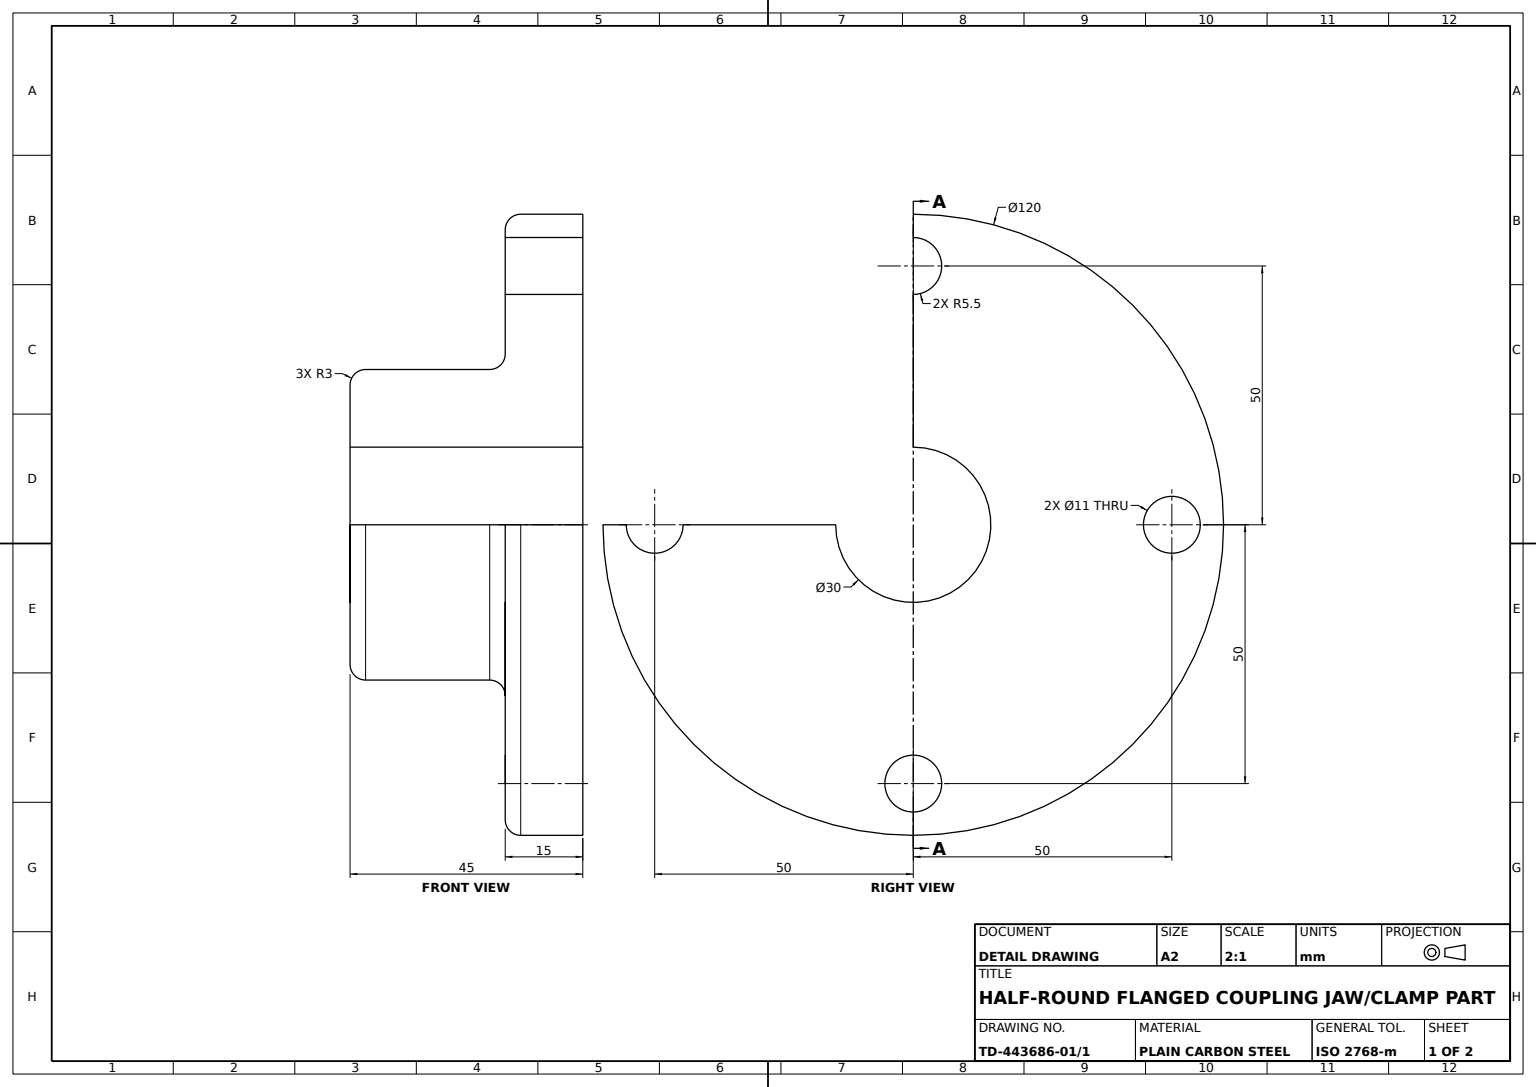
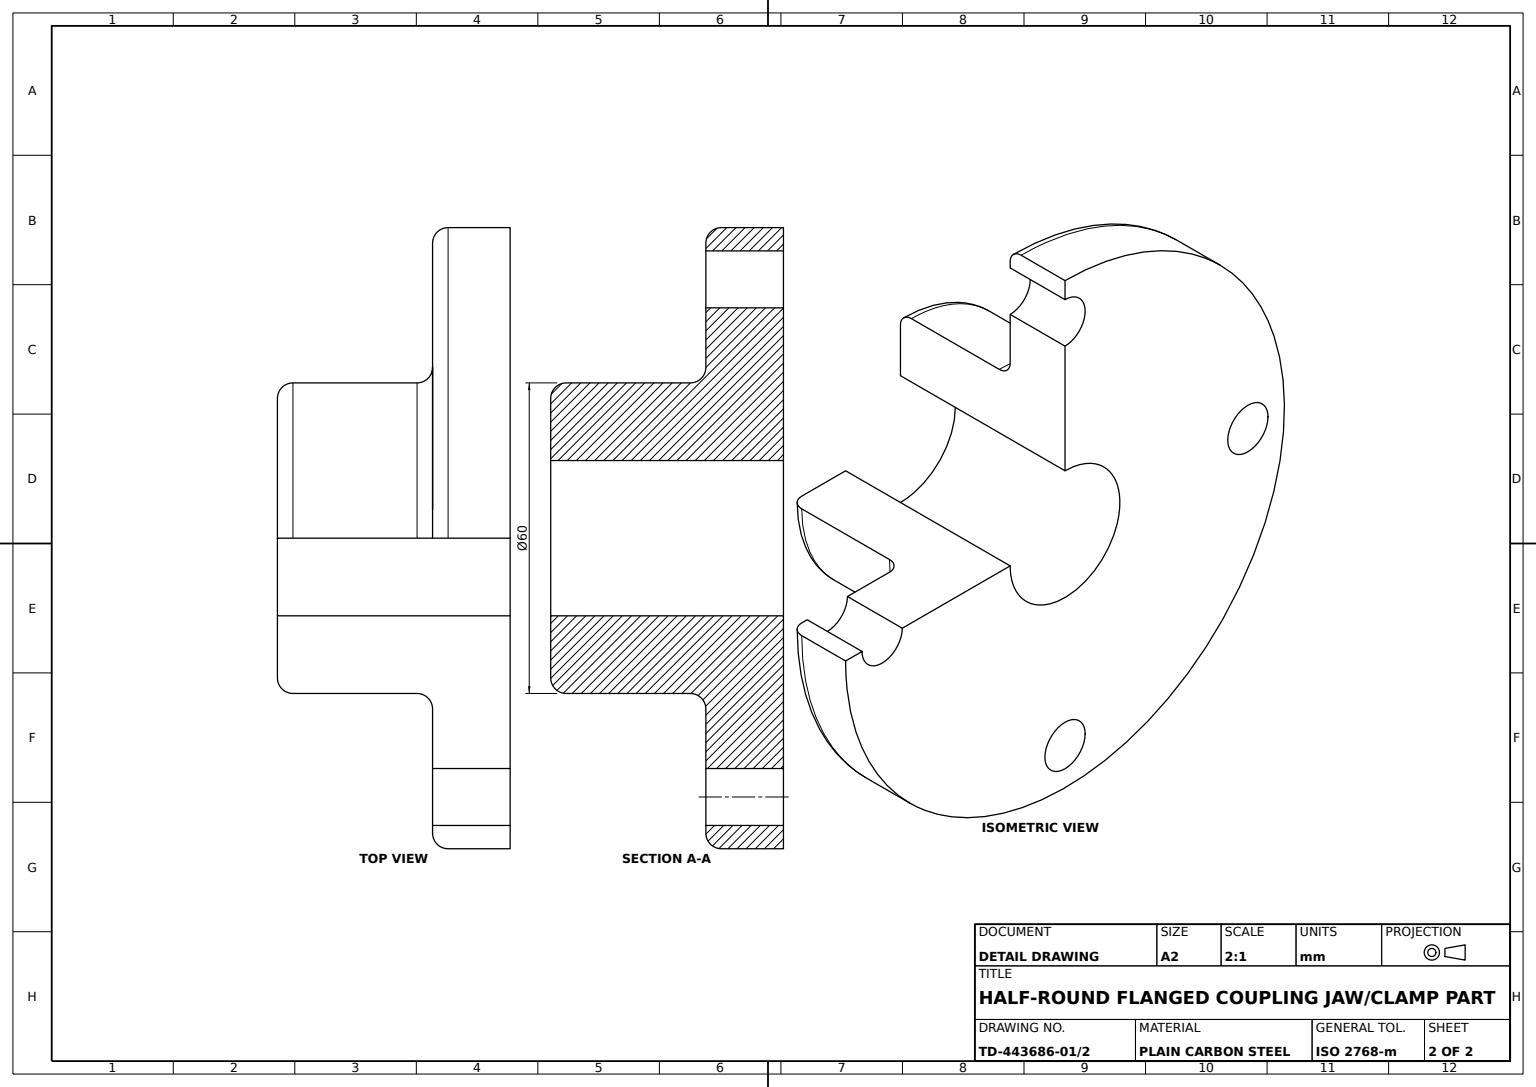
from build123d import *

# Parameters (mm, degrees)
BOLT_HOLES_SKETCH_R = 5.5
BOLT_HOLES_11_DEPTH = 91
EDGE_FILLET_R3_R    = 3
SIDE_CUTOUT_DEPTH   = 97.046863624


with BuildPart() as part:
    # Bed Profile Sketch → Bed Body Revolve (revolve)
    with BuildSketch(Plane.XY, mode=Mode.PRIVATE) as bed_body_revolve_sk:
        Polygon((17.920353982, 15), (17.920353982, 60), (2.920353982, 60), (2.920353982, 30), (-27.079646018, 30), (-27.079646018, 15), align=None)
    revolve(bed_body_revolve_sk.sketch.rotate(Axis((-55.752212389, 0, 0), (1, 0, 0)), 90), axis=Axis((-55.752212389, 0, 0), (1, 0, 0)))

    # Bolt Holes Sketch → Bolt Holes Ø11 (cut, through all)
    with BuildSketch(Plane.ZY.offset(-2.920353982)):
        with Locations((0, 50)):
            Circle(BOLT_HOLES_SKETCH_R)
        with Locations((50, 0)):
            Circle(BOLT_HOLES_SKETCH_R)
        with Locations((0, -50)):
            Circle(BOLT_HOLES_SKETCH_R)
        with Locations((-50, 0)):
            Circle(BOLT_HOLES_SKETCH_R)
    extrude(amount=-BOLT_HOLES_11_DEPTH, mode=Mode.SUBTRACT)

    # Edge Fillet R3
    edge_fillet_r3_edges = [part.edges().sort_by_distance(p)[0] for p in [
        (-27.079646018, 0, -30),
        (2.920353982, 0, -30),
        (2.920353982, 0, -60),
    ]]
    fillet(edge_fillet_r3_edges, radius=EDGE_FILLET_R3_R)

    # Side Cutout Sketch → Side Cutout (cut, through all)
    with BuildSketch(Plane.ZY.offset(27.079646018)):
        with BuildLine():
            Line((0, 77.957463499), (0, 0))
            Line((0, 0), (74.222252728, 0))
            ThreePointArc((74.222252728, 0), (53.256645699, 54.350663604), (0, 77.957463499))
        make_face()
    extrude(amount=-SIDE_CUTOUT_DEPTH, mode=Mode.SUBTRACT)


solid = part.part
